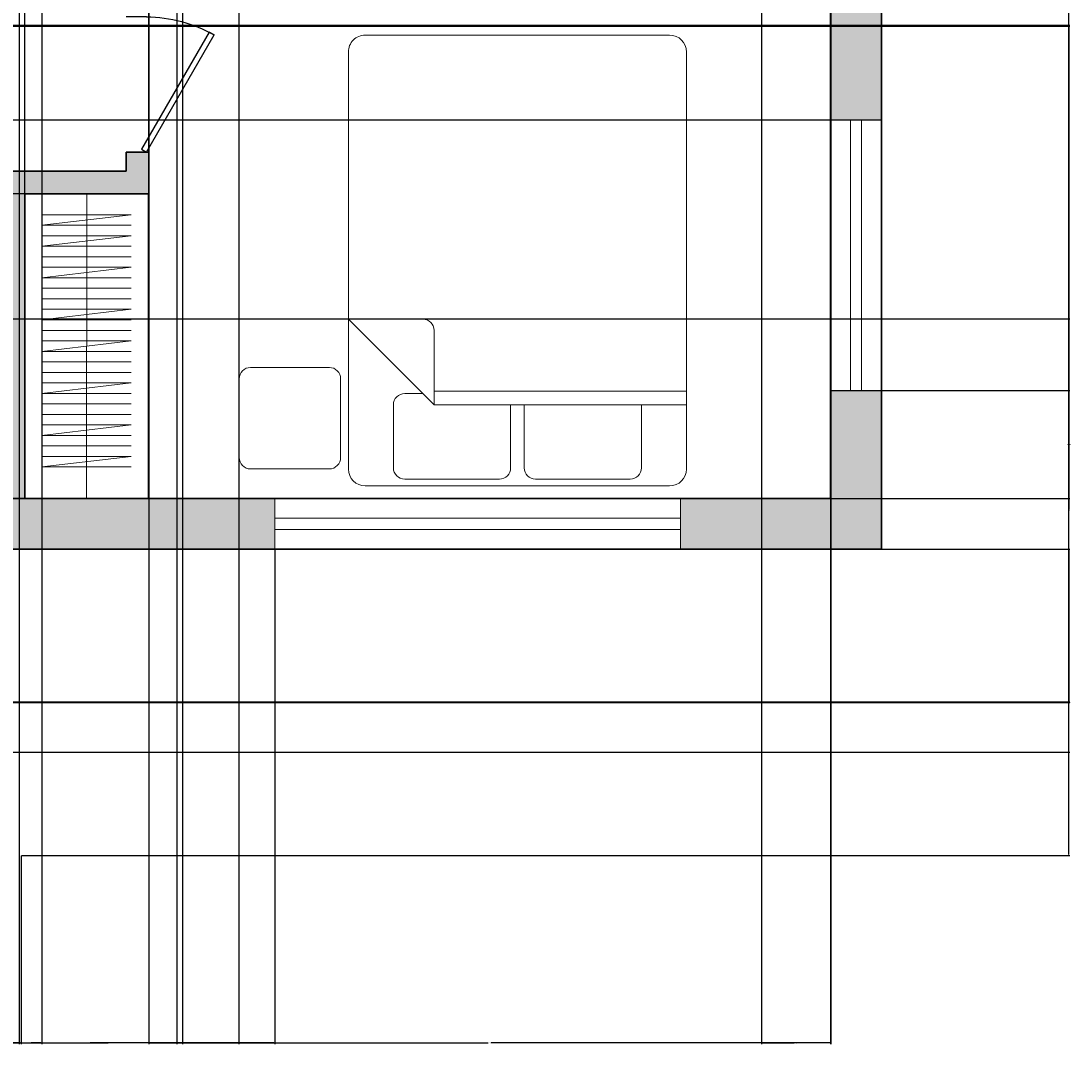
# Model space of a CAD drawing. Units: inches. Extents: x 1531 to 2263, y 2711 to 3216.
# Tile 9 of 12: x 2076 to 2263, y 2711 to 2893. Entities that reach past the tile are written whole.
import ezdxf

# ---------------------------------------------------------------- set-up
doc = ezdxf.new("R2010")
doc.units = ezdxf.units.IN
for name, color, linetype, lineweight in [('A-ANNO-DIMS', 2, 'Continuous', 18), ('A-DOOR', 3, 'Continuous', 25), ('A-FLOR-CASE', 9, 'Continuous', 18), ('A-FURN', 8, 'Continuous', 18), ('A-GLAZ', 4, 'Continuous', 18), ('A-WALL', 7, 'Continuous', 35)]:
    doc.layers.add(name, color=color, linetype=linetype, lineweight=lineweight)
doc.layers.add('A-WALL-PATT', color=18, linetype='Continuous', lineweight=13, true_color=0x000000)
doc.styles.get("Standard").update_dxf_attribs({"font": 'arial.ttf'})
doc.dimstyles.get("Standard").update_dxf_attribs({"dimtxt": 0.18, "dimasz": 0.18, "dimexe": 0.18, "dimexo": 0.0625, "dimgap": 0.09, "dimtad": 0, "dimtih": 1, "dimtoh": 1, "dimdec": 4, "dimzin": 0, "dimdsep": 46, "dimtxsty": 'Standard', "dimcen": 0.09, "dimadec": 0, "dimazin": 0, "dimtfac": 1, "dimtdec": 4, "dimtofl": 0, "dimtmove": 0, "dimatfit": 3, "dimfxl": 1, "dimtolj": 1, "dimtzin": 0, "dimarcsym": 0})

# ---------------------------------------------------------------- blocks, each defined once
blk = doc.blocks.new('*U3')
for p, q in [((0, 0), (0, -6)), ((40, 0), (40, -6))]:
    blk.add_line(p, q)
blk.add_lwpolyline([(0, 0), (34.64, 20), (35.52, 18.48), (0.87, -1.52)], close=True)
blk.add_arc((0, 0), 40, 0, 30)
blk = doc.blocks.new('Bed - Queen')
for p, q in [((3, 0), (57, 0)), ((10, -1.2), (26.8, -1.2)), ((33.2, -1.2), (50, -1.2)), ((0, -77), (0, -3)), ((8, -14.4), (8, -3.2)), ((28.8, -3.2), (28.8, -14.4)), ((31.2, -14.4), (31.2, -3.2)), ((52, -3.2), (52, -14.4)), ((60, -3), (60, -77)), ((0, -14.4), (44.8, -14.4)), ((60, -29.6), (44.8, -14.4)), ((44.8, -14.4), (44.8, -27.6)), ((50, -16.4), (46.8, -16.4)), ((44.8, -16.8), (0, -16.8)), ((46.8, -29.6), (60, -29.6)), ((57, -80), (3, -80))]:
    blk.add_line(p, q)
blk.add_lwpolyline([(63.37, -3.02), (77.37, -3.02, -0.414214), (79.37, -5.02), (79.37, -19.02, -0.414214), (77.37, -21.02), (63.37, -21.02, -0.414214), (61.37, -19.02), (61.37, -5.02, -0.414214)], format="xyb", close=True)
for centre, radius, start, end in [((3, -3), 3, 90, 180), ((57, -3), 3, 0, 90), ((10, -3.2), 2, 90, 180), ((26.8, -3.2), 2, 0, 90), ((33.2, -3.2), 2, 90, 180), ((50, -3.2), 2, 0, 90), ((50, -14.4), 2, 270, 0), ((46.8, -27.6), 2, 180, 270), ((3, -77), 3, 180, 270), ((57, -77), 3, 270, 0)]:
    blk.add_arc(centre, radius, start, end)
blk = doc.blocks.new('WIN-72IN')
for p, q in [((0, 5.5), (72, 5.5)), ((0, 3.5), (72, 3.5))]:
    blk.add_line(p, q)
for points in [[(0, 9), (0, 0)], [(72, 0), (72, 9)]]:
    blk.add_lwpolyline(points)
blk = doc.blocks.new('WIN-48IN')
for p, q in [((3.5, 48), (3.5, 0)), ((5.5, 48), (5.5, 0))]:
    blk.add_line(p, q)
for points in [[(0, 48), (9, 48)], [(9, 0), (0, 0)]]:
    blk.add_lwpolyline(points)
blk = doc.blocks.new('*D55')
at = {"layer": 'A-ANNO-DIMS', "color": 0, "lineweight": -2, "transparency": 16777216}
for p, q in [((2228.97, 3183.02), (2262.37, 3183.02)), ((2262.19, 3182.84), (2262.19, 2963.95)), ((2262.19, 2744.7), (2262.19, 2963.59)), ((2076.3, 2744.52), (2262.37, 2744.52))]:
    blk.add_line(p, q, dxfattribs=at)
at = {"layer": 'A-ANNO-DIMS', "color": 0, "transparency": 16777216}
for points in [[(2262.16, 3182.84), (2262.22, 3182.84), (2262.19, 3183.02)], [(2262.16, 2744.7), (2262.22, 2744.7), (2262.19, 2744.52)]]:
    blk.add_solid(points, dxfattribs=at)
at = {"layer": 'Defpoints', "color": 0, "transparency": 16777216}
for p in [(2228.91, 3183.02), (2076.24, 2744.52), (2262.19, 2744.52)]:
    blk.add_point(p, dxfattribs=at)
at = {"layer": 'A-ANNO-DIMS', "color": 0, "transparency": 16777216, "insert": (2262.19, 2963.77), "char_height": 0.18, "attachment_point": 5}
blk.add_mtext('\\A1;438.5', dxfattribs=at)
blk = doc.blocks.new('*D65')
at = {"layer": 'A-ANNO-DIMS', "color": 0, "lineweight": -2, "transparency": 16777216}
for p, q in [((1577.97, 2891.68), (2262.37, 2891.68)), ((2262.19, 2891.5), (2262.19, 2831.86)), ((2262.19, 2771.86), (2262.19, 2831.5)), ((1577.97, 2771.68), (2262.37, 2771.68))]:
    blk.add_line(p, q, dxfattribs=at)
at = {"layer": 'A-ANNO-DIMS', "color": 0, "transparency": 16777216}
for points in [[(2262.16, 2891.5), (2262.22, 2891.5), (2262.19, 2891.68)], [(2262.16, 2771.86), (2262.22, 2771.86), (2262.19, 2771.68)]]:
    blk.add_solid(points, dxfattribs=at)
at = {"layer": 'Defpoints', "color": 0, "transparency": 16777216}
for p in [(1577.91, 2891.68), (1577.91, 2771.68), (2262.19, 2771.68)]:
    blk.add_point(p, dxfattribs=at)
at = {"layer": 'A-ANNO-DIMS', "color": 0, "transparency": 16777216, "insert": (2262.19, 2831.68), "char_height": 0.18, "attachment_point": 5}
blk.add_mtext('\\A1;120', dxfattribs=at)
blk = doc.blocks.new('*D70')
at = {"layer": 'A-ANNO-DIMS', "color": 0, "lineweight": -2, "transparency": 16777216}
for p, q in [((1736.97, 2839.76), (2262.37, 2839.76)), ((2262.19, 2839.58), (2262.19, 2805.94)), ((2262.19, 2771.94), (2262.19, 2805.58)), ((1736.97, 2771.76), (2262.37, 2771.76))]:
    blk.add_line(p, q, dxfattribs=at)
at = {"layer": 'A-ANNO-DIMS', "color": 0, "transparency": 16777216}
for points in [[(2262.16, 2839.58), (2262.22, 2839.58), (2262.19, 2839.76)], [(2262.16, 2771.94), (2262.22, 2771.94), (2262.19, 2771.76)]]:
    blk.add_solid(points, dxfattribs=at)
at = {"layer": 'Defpoints', "color": 0, "transparency": 16777216}
for p in [(1736.91, 2839.76), (2262.19, 2839.76), (1736.91, 2771.76)]:
    blk.add_point(p, dxfattribs=at)
at = {"layer": 'A-ANNO-DIMS', "color": 0, "transparency": 16777216, "insert": (2262.19, 2805.76), "char_height": 0.18, "attachment_point": 5}
blk.add_mtext('\\A1;68', dxfattribs=at)
blk = doc.blocks.new('*D72')
at = {"layer": 'A-ANNO-DIMS', "color": 0, "lineweight": -2, "transparency": 16777216}
for p, q in [((1986.65, 2744.45), (1986.65, 2711.06)), ((2076.24, 2744.45), (2076.24, 2711.06)), ((1986.83, 2711.24), (2031.05, 2711.24)), ((2076.06, 2711.24), (2031.84, 2711.24))]:
    blk.add_line(p, q, dxfattribs=at)
at = {"layer": 'A-ANNO-DIMS', "color": 0, "transparency": 16777216}
for points in [[(1986.83, 2711.27), (1986.83, 2711.21), (1986.65, 2711.24)], [(2076.06, 2711.27), (2076.06, 2711.21), (2076.24, 2711.24)]]:
    blk.add_solid(points, dxfattribs=at)
at = {"layer": 'Defpoints', "color": 0, "transparency": 16777216}
for p in [(1986.65, 2744.52), (2076.24, 2744.52), (2076.24, 2711.24)]:
    blk.add_point(p, dxfattribs=at)
at = {"layer": 'A-ANNO-DIMS', "color": 0, "transparency": 16777216, "insert": (2031.44, 2711.24), "char_height": 0.18, "attachment_point": 5}
blk.add_mtext('\\A1;89.59', dxfattribs=at)
blk = doc.blocks.new('*D73')
at = {"layer": 'A-ANNO-DIMS', "color": 0, "lineweight": -2, "transparency": 16777216}
for p, q in [((2076.3, 2798.86), (2262.37, 2798.86)), ((2262.19, 2798.68), (2262.19, 2771.87)), ((2262.19, 2744.7), (2262.19, 2771.51)), ((2076.3, 2744.52), (2262.37, 2744.52))]:
    blk.add_line(p, q, dxfattribs=at)
at = {"layer": 'A-ANNO-DIMS', "color": 0, "transparency": 16777216}
for points in [[(2262.16, 2798.68), (2262.22, 2798.68), (2262.19, 2798.86)], [(2262.16, 2744.7), (2262.22, 2744.7), (2262.19, 2744.52)]]:
    blk.add_solid(points, dxfattribs=at)
at = {"layer": 'Defpoints', "color": 0, "transparency": 16777216}
for p in [(2076.24, 2798.86), (2262.19, 2798.86), (2076.24, 2744.52)]:
    blk.add_point(p, dxfattribs=at)
at = {"layer": 'A-ANNO-DIMS', "color": 0, "transparency": 16777216, "insert": (2262.19, 2771.69), "char_height": 0.18, "attachment_point": 5}
blk.add_mtext('\\A1;54.35', dxfattribs=at)
blk = doc.blocks.new('*D74')
at = {"layer": 'A-ANNO-DIMS', "color": 0, "lineweight": -2, "transparency": 16777216}
for p, q in [((2098.91, 2899.27), (2098.91, 2711.06)), ((2219.91, 2899.33), (2219.91, 2711.06)), ((2099.09, 2711.24), (2159.15, 2711.24)), ((2219.73, 2711.24), (2159.67, 2711.24))]:
    blk.add_line(p, q, dxfattribs=at)
at = {"layer": 'A-ANNO-DIMS', "color": 0, "transparency": 16777216}
for points in [[(2099.09, 2711.27), (2099.09, 2711.21), (2098.91, 2711.24)], [(2219.73, 2711.27), (2219.73, 2711.21), (2219.91, 2711.24)]]:
    blk.add_solid(points, dxfattribs=at)
at = {"layer": 'Defpoints', "color": 0, "transparency": 16777216}
for p in [(2098.91, 2899.33), (2219.91, 2899.4), (2219.91, 2711.24)]:
    blk.add_point(p, dxfattribs=at)
at = {"layer": 'A-ANNO-DIMS', "color": 0, "transparency": 16777216, "insert": (2159.41, 2711.24), "char_height": 0.18, "attachment_point": 5}
blk.add_mtext('\\A1;121', dxfattribs=at)
blk = doc.blocks.new('*D75')
at = {"layer": 'A-ANNO-DIMS', "color": 0, "lineweight": -2, "transparency": 16777216}
for p, q in [((2219.85, 2899.4), (1531.04, 2899.4)), ((1531.22, 2899.22), (1531.22, 2853.81)), ((1531.22, 2808.04), (1531.22, 2853.45)), ((2219.85, 2807.86), (1531.04, 2807.86))]:
    blk.add_line(p, q, dxfattribs=at)
at = {"layer": 'A-ANNO-DIMS', "color": 0, "transparency": 16777216}
for points in [[(1531.19, 2899.22), (1531.25, 2899.22), (1531.22, 2899.4)], [(1531.19, 2808.04), (1531.25, 2808.04), (1531.22, 2807.86)]]:
    blk.add_solid(points, dxfattribs=at)
at = {"layer": 'Defpoints', "color": 0, "transparency": 16777216}
for p in [(1531.22, 2899.4), (2219.91, 2899.4), (2219.91, 2807.86)]:
    blk.add_point(p, dxfattribs=at)
at = {"layer": 'A-ANNO-DIMS', "color": 0, "transparency": 16777216, "insert": (1531.22, 2853.63), "char_height": 0.18, "attachment_point": 5}
blk.add_mtext('\\A1;91.53', dxfattribs=at)
blk = doc.blocks.new('*D81')
at = {"layer": 'A-ANNO-DIMS', "color": 0, "lineweight": -2, "transparency": 16777216}
for p, q in [((1933.97, 2891.87), (2262.37, 2891.87)), ((2262.19, 2891.69), (2262.19, 2850.05)), ((2262.19, 2808.04), (2262.19, 2849.68)), ((1933.97, 2807.86), (2262.37, 2807.86))]:
    blk.add_line(p, q, dxfattribs=at)
at = {"layer": 'A-ANNO-DIMS', "color": 0, "transparency": 16777216}
for points in [[(2262.16, 2891.69), (2262.22, 2891.69), (2262.19, 2891.87)], [(2262.16, 2808.04), (2262.22, 2808.04), (2262.19, 2807.86)]]:
    blk.add_solid(points, dxfattribs=at)
at = {"layer": 'Defpoints', "color": 0, "transparency": 16777216}
for p in [(1933.91, 2891.87), (2262.19, 2891.87), (1933.91, 2807.86)]:
    blk.add_point(p, dxfattribs=at)
at = {"layer": 'A-ANNO-DIMS', "color": 0, "transparency": 16777216, "insert": (2262.19, 2849.86), "char_height": 0.18, "attachment_point": 5}
blk.add_mtext('\\A1;84', dxfattribs=at)
blk = doc.blocks.new('*D84')
at = {"layer": 'A-ANNO-DIMS', "color": 0, "lineweight": -2, "transparency": 16777216}
for p, q in [((2079.91, 3089.28), (2079.91, 2711.06)), ((2103.91, 3089.28), (2103.91, 2711.06)), ((2080.09, 2711.24), (2091.69, 2711.24)), ((2103.73, 2711.24), (2092.13, 2711.24))]:
    blk.add_line(p, q, dxfattribs=at)
at = {"layer": 'A-ANNO-DIMS', "color": 0, "transparency": 16777216}
for points in [[(2080.09, 2711.27), (2080.09, 2711.21), (2079.91, 2711.24)], [(2103.73, 2711.27), (2103.73, 2711.21), (2103.91, 2711.24)]]:
    blk.add_solid(points, dxfattribs=at)
at = {"layer": 'Defpoints', "color": 0, "transparency": 16777216}
for p in [(2079.91, 3089.34), (2103.91, 3089.34), (2103.91, 2711.24)]:
    blk.add_point(p, dxfattribs=at)
at = {"layer": 'A-ANNO-DIMS', "color": 0, "transparency": 16777216, "insert": (2091.91, 2711.24), "char_height": 0.18, "attachment_point": 5}
blk.add_mtext('\\A1;24', dxfattribs=at)
blk = doc.blocks.new('*D97')
at = {"layer": 'A-ANNO-DIMS', "color": 0, "lineweight": -2, "transparency": 16777216}
for p, q in [((2054.91, 2798.8), (2054.91, 2711.06)), ((2121.28, 2798.8), (2121.28, 2711.06)), ((2055.09, 2711.24), (2087.7, 2711.24)), ((2121.09, 2711.24), (2088.49, 2711.24))]:
    blk.add_line(p, q, dxfattribs=at)
at = {"layer": 'A-ANNO-DIMS', "color": 0, "transparency": 16777216}
for points in [[(2055.09, 2711.27), (2055.09, 2711.21), (2054.91, 2711.24)], [(2121.09, 2711.27), (2121.09, 2711.21), (2121.28, 2711.24)]]:
    blk.add_solid(points, dxfattribs=at)
at = {"layer": 'Defpoints', "color": 0, "transparency": 16777216}
for p in [(2054.91, 2798.86), (2121.28, 2798.86), (2054.91, 2711.24)]:
    blk.add_point(p, dxfattribs=at)
at = {"layer": 'A-ANNO-DIMS', "color": 0, "transparency": 16777216, "insert": (2088.09, 2711.24), "char_height": 0.18, "attachment_point": 5}
blk.add_mtext('\\A1;66.36', dxfattribs=at)
blk = doc.blocks.new('*D101')
at = {"layer": 'A-ANNO-DIMS', "color": 0, "lineweight": -2, "transparency": 16777216}
for p, q in [((2228.85, 2918.81), (1531.04, 2918.81)), ((1531.22, 2918.63), (1531.22, 2897.08)), ((1531.22, 2875.18), (1531.22, 2896.72)), ((2228.85, 2875), (1531.04, 2875))]:
    blk.add_line(p, q, dxfattribs=at)
at = {"layer": 'A-ANNO-DIMS', "color": 0, "transparency": 16777216}
for points in [[(1531.19, 2918.63), (1531.25, 2918.63), (1531.22, 2918.81)], [(1531.19, 2875.18), (1531.25, 2875.18), (1531.22, 2875)]]:
    blk.add_solid(points, dxfattribs=at)
at = {"layer": 'Defpoints', "color": 0, "transparency": 16777216}
for p in [(2228.91, 2918.81), (1531.22, 2875), (2228.91, 2875)]:
    blk.add_point(p, dxfattribs=at)
at = {"layer": 'A-ANNO-DIMS', "color": 0, "transparency": 16777216, "insert": (1531.22, 2896.9), "char_height": 0.18, "attachment_point": 5}
blk.add_mtext('\\A1;43.81', dxfattribs=at)
blk = doc.blocks.new('*D102')
at = {"layer": 'A-ANNO-DIMS', "color": 0, "lineweight": -2, "transparency": 16777216}
for p, q in [((2219.97, 2827), (2262.37, 2827)), ((2262.19, 2826.82), (2262.19, 2817.61)), ((2262.19, 2808.04), (2262.19, 2817.25)), ((2219.97, 2807.86), (2262.37, 2807.86))]:
    blk.add_line(p, q, dxfattribs=at)
at = {"layer": 'A-ANNO-DIMS', "color": 0, "transparency": 16777216}
for points in [[(2262.16, 2826.82), (2262.22, 2826.82), (2262.19, 2827)], [(2262.16, 2808.04), (2262.22, 2808.04), (2262.19, 2807.86)]]:
    blk.add_solid(points, dxfattribs=at)
at = {"layer": 'Defpoints', "color": 0, "transparency": 16777216}
for p in [(2219.91, 2827), (2262.19, 2827), (2219.91, 2807.86)]:
    blk.add_point(p, dxfattribs=at)
at = {"layer": 'A-ANNO-DIMS', "color": 0, "transparency": 16777216, "insert": (2262.19, 2817.43), "char_height": 0.18, "attachment_point": 5}
blk.add_mtext('\\A1;19.133', dxfattribs=at)
blk = doc.blocks.new('*D105')
at = {"layer": 'A-ANNO-DIMS', "color": 0, "lineweight": -2, "transparency": 16777216}
for p, q in [((2104.87, 2975.27), (2104.87, 2711.06)), ((2114.87, 2975.27), (2114.87, 2711.06)), ((2105.05, 2711.24), (2109.66, 2711.24)), ((2114.69, 2711.24), (2110.08, 2711.24))]:
    blk.add_line(p, q, dxfattribs=at)
at = {"layer": 'A-ANNO-DIMS', "color": 0, "transparency": 16777216}
for points in [[(2105.05, 2711.27), (2105.05, 2711.21), (2104.87, 2711.24)], [(2114.69, 2711.27), (2114.69, 2711.21), (2114.87, 2711.24)]]:
    blk.add_solid(points, dxfattribs=at)
at = {"layer": 'Defpoints', "color": 0, "transparency": 16777216}
for p in [(2104.87, 2975.33), (2114.87, 2975.33), (2114.87, 2711.24)]:
    blk.add_point(p, dxfattribs=at)
at = {"layer": 'A-ANNO-DIMS', "color": 0, "transparency": 16777216, "insert": (2109.87, 2711.24), "char_height": 0.18, "attachment_point": 5}
blk.add_mtext('\\A1;10', dxfattribs=at)
blk = doc.blocks.new('*D108')
at = {"layer": 'A-ANNO-DIMS', "color": 0, "lineweight": -2, "transparency": 16777216}
for p, q in [((1933.97, 2798.86), (2262.37, 2798.86)), ((2262.19, 2798.68), (2262.19, 2781.05)), ((2262.19, 2763.05), (2262.19, 2780.68)), ((1933.97, 2762.87), (2262.37, 2762.87))]:
    blk.add_line(p, q, dxfattribs=at)
at = {"layer": 'A-ANNO-DIMS', "color": 0, "transparency": 16777216}
for points in [[(2262.16, 2798.68), (2262.22, 2798.68), (2262.19, 2798.86)], [(2262.16, 2763.05), (2262.22, 2763.05), (2262.19, 2762.87)]]:
    blk.add_solid(points, dxfattribs=at)
at = {"layer": 'Defpoints', "color": 0, "transparency": 16777216}
for p in [(1933.91, 2798.86), (2262.19, 2798.86), (1933.91, 2762.87)]:
    blk.add_point(p, dxfattribs=at)
at = {"layer": 'A-ANNO-DIMS', "color": 0, "transparency": 16777216, "insert": (2262.19, 2780.86), "char_height": 0.18, "attachment_point": 5}
blk.add_mtext('\\A1;36', dxfattribs=at)
blk = doc.blocks.new('*D123')
at = {"layer": 'A-ANNO-DIMS', "color": 0, "lineweight": -2, "transparency": 16777216}
for p, q in [((2207.66, 3152.42), (2207.66, 2711.06)), ((2219.92, 3149.95), (2219.92, 2711.06)), ((2207.84, 2711.24), (2213.41, 2711.24)), ((2219.74, 2711.24), (2214.18, 2711.24))]:
    blk.add_line(p, q, dxfattribs=at)
at = {"layer": 'A-ANNO-DIMS', "color": 0, "transparency": 16777216}
for points in [[(2207.84, 2711.27), (2207.84, 2711.21), (2207.66, 2711.24)], [(2219.74, 2711.27), (2219.74, 2711.21), (2219.92, 2711.24)]]:
    blk.add_solid(points, dxfattribs=at)
at = {"layer": 'Defpoints', "color": 0, "transparency": 16777216}
for p in [(2207.66, 3152.48), (2219.92, 3150.02), (2207.66, 2711.24)]:
    blk.add_point(p, dxfattribs=at)
at = {"layer": 'A-ANNO-DIMS', "color": 0, "transparency": 16777216, "insert": (2213.79, 2711.24), "char_height": 0.18, "attachment_point": 5}
blk.add_mtext('\\A1;12.26', dxfattribs=at)
blk = doc.blocks.new('*D124')
at = {"layer": 'A-ANNO-DIMS', "color": 0, "lineweight": -2, "transparency": 16777216}
for p, q in [((2076.91, 2862.01), (2076.91, 3216.47)), ((2077.09, 3216.29), (2087.69, 3216.29)), ((2098.73, 3216.29), (2088.13, 3216.29)), ((2098.91, 2862.01), (2098.91, 3216.47))]:
    blk.add_line(p, q, dxfattribs=at)
at = {"layer": 'A-ANNO-DIMS', "color": 0, "transparency": 16777216}
for points in [[(2077.09, 3216.32), (2077.09, 3216.26), (2076.91, 3216.29)], [(2098.73, 3216.32), (2098.73, 3216.26), (2098.91, 3216.29)]]:
    blk.add_solid(points, dxfattribs=at)
at = {"layer": 'Defpoints', "color": 0, "transparency": 16777216}
for p in [(2076.91, 3216.29), (2076.91, 2861.95), (2098.91, 2861.95)]:
    blk.add_point(p, dxfattribs=at)
at = {"layer": 'A-ANNO-DIMS', "color": 0, "transparency": 16777216, "insert": (2087.91, 3216.29), "char_height": 0.18, "attachment_point": 5}
blk.add_mtext('\\A1;22', dxfattribs=at)
blk = doc.blocks.new('*D125')
at = {"layer": 'A-ANNO-DIMS', "color": 0, "lineweight": -2, "transparency": 16777216}
for p, q in [((2076.85, 2861.95), (1531.04, 2861.95)), ((1531.22, 2861.77), (1531.22, 2835.09)), ((1531.22, 2808.04), (1531.22, 2834.72)), ((2076.85, 2807.86), (1531.04, 2807.86))]:
    blk.add_line(p, q, dxfattribs=at)
at = {"layer": 'A-ANNO-DIMS', "color": 0, "transparency": 16777216}
for points in [[(1531.19, 2861.77), (1531.25, 2861.77), (1531.22, 2861.95)], [(1531.19, 2808.04), (1531.25, 2808.04), (1531.22, 2807.86)]]:
    blk.add_solid(points, dxfattribs=at)
at = {"layer": 'Defpoints', "color": 0, "transparency": 16777216}
for p in [(2076.91, 2861.95), (1531.22, 2807.86), (2076.91, 2807.86)]:
    blk.add_point(p, dxfattribs=at)
at = {"layer": 'A-ANNO-DIMS', "color": 0, "transparency": 16777216, "insert": (1531.22, 2834.91), "char_height": 0.18, "attachment_point": 5}
blk.add_mtext('\\A1;54.09', dxfattribs=at)
blk = doc.blocks.new('*D130')
at = {"layer": 'A-ANNO-DIMS', "color": 0, "lineweight": -2, "transparency": 16777216}
for p, q in [((2075.91, 3029.88), (2075.91, 2711.06)), ((2079.91, 3025.88), (2079.91, 2711.06)), ((2076.09, 2711.24), (2077.76, 2711.24)), ((2079.73, 2711.24), (2078.06, 2711.24))]:
    blk.add_line(p, q, dxfattribs=at)
at = {"layer": 'A-ANNO-DIMS', "color": 0, "transparency": 16777216}
for points in [[(2076.09, 2711.27), (2076.09, 2711.21), (2075.91, 2711.24)], [(2079.73, 2711.27), (2079.73, 2711.21), (2079.91, 2711.24)]]:
    blk.add_solid(points, dxfattribs=at)
at = {"layer": 'Defpoints', "color": 0, "transparency": 16777216}
for p in [(2075.91, 3029.94), (2079.91, 3025.94), (2075.91, 2711.24)]:
    blk.add_point(p, dxfattribs=at)
at = {"layer": 'A-ANNO-DIMS', "color": 0, "transparency": 16777216, "insert": (2077.91, 2711.24), "char_height": 0.18, "attachment_point": 5}
blk.add_mtext('\\A1;4', dxfattribs=at)

msp = doc.modelspace()

# ---------------------------------------------------------------- hatches: boundary and pattern name
at = {"layer": 'A-WALL-PATT'}
h = msp.add_hatch(color=256, dxfattribs=at)
h.dxf.hatch_style = 1
h.paths.add_polyline_path([(2228.9101, 2918.8056), (2219.9101, 2918.8056), (2219.9101, 2903.3968), (2213.9101, 2903.3937), (2213.9101, 2899.3968), (2219.9101, 2899.3968), (2219.9101, 2874.9957), (2228.9101, 2874.9957)])
h = msp.add_hatch(color=256, dxfattribs=at)
h.dxf.hatch_style = 1
h.paths.add_polyline_path([(2121.275, 2807.8631), (2076.9101, 2807.8631), (2076.9101, 2861.9499), (2098.9101, 2861.9499), (2098.9101, 2869.3336), (2094.9101, 2869.3336), (2094.9101, 2865.9499), (2072.9101, 2865.9499), (2072.9101, 2807.8631), (2054.9101, 2807.8631), (2054.9101, 2798.8631), (2121.275, 2798.8631)])
h = msp.add_hatch(color=256, dxfattribs=at)
h.dxf.hatch_style = 1
h.paths.add_polyline_path([(2228.9101, 2826.9957), (2219.9101, 2826.9957), (2219.9101, 2807.8631), (2193.275, 2807.8631), (2193.275, 2798.8631), (2228.9101, 2798.8631)])

# ---------------------------------------------------------------- linework, layer by layer
at = {"layer": 'A-FLOR-CASE'}
for p, q in [((2076.9101, 2861.9499), (2098.7759, 2861.9499)), ((2076.9101, 2807.8631), (2076.9101, 2861.9499)), ((2087.9101, 2861.9499), (2087.843, 2807.8631)), ((2098.7759, 2861.9499), (2098.7759, 2807.8631)), ((2076.905, 2860.0848), (2076.9101, 2860.0848)), ((2076.8998, 2858.2197), (2076.9101, 2858.2197)), ((2079.9101, 2858.2197), (2095.7759, 2858.2197)), ((2095.7759, 2858.2197), (2079.9101, 2856.3545)), ((2076.8946, 2856.3545), (2076.9101, 2856.3545)), ((2079.9101, 2856.3545), (2095.7759, 2856.3545)), ((2079.9101, 2854.4894), (2095.7759, 2854.4894)), ((2095.7759, 2854.4894), (2079.9101, 2852.6243)), ((2079.9101, 2852.6243), (2095.7759, 2852.6243)), ((2079.9101, 2850.7591), (2095.7759, 2850.7591)), ((2079.9101, 2848.894), (2095.7759, 2848.894)), ((2095.7759, 2848.894), (2079.9101, 2847.0289)), ((2079.9101, 2847.0289), (2095.7759, 2847.0289)), ((2079.9101, 2845.1637), (2095.7759, 2845.1637)), ((2079.9101, 2843.2986), (2095.7759, 2843.2986)), ((2079.9101, 2841.4335), (2095.7759, 2841.4335)), ((2095.7759, 2841.4335), (2079.9101, 2839.5683)), ((2079.9101, 2839.5683), (2095.7759, 2839.5683)), ((2079.9101, 2837.7032), (2095.7759, 2837.7032)), ((2079.9101, 2835.838), (2095.7759, 2835.838)), ((2095.7759, 2835.838), (2079.9101, 2833.9729)), ((2079.9101, 2833.9729), (2095.7759, 2833.9729)), ((2079.9101, 2832.1078), (2095.7759, 2832.1078)), ((2079.9101, 2830.2426), (2095.7759, 2830.2426)), ((2079.9101, 2828.3775), (2095.7759, 2828.3775)), ((2095.7759, 2828.3775), (2079.9101, 2826.5124)), ((2079.9101, 2826.5124), (2095.7759, 2826.5124)), ((2079.9101, 2824.6472), (2095.7759, 2824.6472)), ((2079.9101, 2822.7821), (2095.7759, 2822.7821)), ((2079.9101, 2820.917), (2095.7759, 2820.917)), ((2095.7759, 2820.917), (2079.9101, 2819.0518)), ((2079.9101, 2819.0518), (2095.7759, 2819.0518)), ((2079.9101, 2817.1867), (2095.7759, 2817.1867)), ((2079.9101, 2815.3216), (2095.7759, 2815.3216)), ((2095.7759, 2815.3216), (2079.9101, 2813.4564)), ((2079.9101, 2813.4564), (2095.7759, 2813.4564)), ((2098.7759, 2807.8631), (2076.9101, 2807.8631))]:
    msp.add_line(p, q, dxfattribs=at)
at = {"layer": 'A-WALL'}
for p, q in [((2219.9101, 2899.3968), (2219.9101, 2807.8631)), ((2098.9101, 2869.3336), (2094.9101, 2869.3336)), ((2094.9101, 2869.3336), (2094.9101, 2865.9499)), ((2098.9101, 2869.3336), (2098.9101, 2861.9499)), ((2094.9258, 2865.9499), (2072.9101, 2865.9499)), ((2094.9101, 2865.9499), (2094.9248, 2865.9499)), ((2094.9237, 2865.9499), (2094.9248, 2865.9499)), ((2098.9101, 2865.952), (2098.9237, 2865.952)), ((2098.9101, 2861.9499), (2076.9101, 2861.9499)), ((2076.9101, 2861.9499), (2076.9101, 2807.8631)), ((2098.9101, 2861.952), (2098.9258, 2861.952)), ((2076.9101, 2807.8631), (2219.9101, 2807.8631)), ((2054.9101, 2798.8631), (2228.9101, 2798.8631))]:
    msp.add_line(p, q, dxfattribs=at)
msp.add_lwpolyline([(1933.9101, 2762.8657), (1568.9111, 2762.6748), (1568.9111, 3182.6749), (2228.9101, 3183.02), (2228.9101, 2798.8631)], dxfattribs=at)

# ---------------------------------------------------------------- block references
at = {"layer": 'A-DOOR', "xscale": -0.6, "yscale": 0.6, "zscale": 0.6, "rotation": 270}
msp.add_blockref('*U3', (2098.5101, 2869.3336), dxfattribs=at)
at = {"layer": 'A-FURN', "rotation": 180}
msp.add_blockref('Bed - Queen', (2194.3244, 2810.0977), dxfattribs=at)
at = {"layer": 'A-GLAZ'}
for name, p in [('WIN-48IN', (2219.9101, 2826.9962)), ('WIN-72IN', (2121.2751, 2798.8631))]:
    msp.add_blockref(name, p, dxfattribs=at)

# ---------------------------------------------------------------- dimensions: what is measured, and where the dimension line sits
at = {"layer": 'A-ANNO-DIMS'}
for base, p1, p2, override, picture, middle in [((2076.9101, 3216.295), (2098.9101, 2861.9499), (2076.9101, 2861.9499), {"dimdec": 0, "dimlfac": 1, "dimrnd": 0, "dimzin": 0, "dimdsep": 46, "dimlunit": 2}, '*D124', (2087.9101, 3216.295)), ((2207.6621, 2711.2407), (2219.9227, 3150.0153), (2207.6621, 3152.4778), {"dimdec": 2, "dimlfac": 1, "dimrnd": 0, "dimzin": 0, "dimdsep": 46, "dimlunit": 2}, '*D123', (2213.7924, 2711.2407)), ((2103.9101, 2711.2407), (2079.9101, 3089.343), (2103.9101, 3089.343), {"dimdec": 0, "dimlfac": 1, "dimrnd": 0, "dimzin": 0, "dimdsep": 46, "dimlunit": 2}, '*D84', (2091.9101, 2711.2407)), ((2075.9101, 2711.2407), (2079.9101, 3025.9421), (2075.9101, 3029.94), {"dimdec": 0, "dimlfac": 1, "dimrnd": 0, "dimzin": 0, "dimdsep": 46, "dimlunit": 2}, '*D130', (2077.9101, 2711.2407)), ((2114.8725, 2711.2407), (2104.8725, 2975.3315), (2114.8725, 2975.3315), {"dimdec": 0, "dimlfac": 1, "dimrnd": 0, "dimzin": 0, "dimdsep": 46, "dimlunit": 2}, '*D105', (2109.8725, 2711.2407)), ((2219.9101, 2711.2407), (2098.9101, 2899.3336), (2219.9101, 2899.3968), {"dimdec": 0, "dimlfac": 1, "dimrnd": 0, "dimzin": 0, "dimdsep": 46, "dimlunit": 2}, '*D74', (2159.4101, 2711.2407)), ((2054.9101, 2711.2407), (2121.275, 2798.8631), (2054.9101, 2798.8631), {"dimdec": 2, "dimlfac": 1, "dimrnd": 0, "dimzin": 0, "dimdsep": 46, "dimlunit": 2}, '*D97', (2088.0926, 2711.2407)), ((2076.2365, 2711.2407), (1986.6484, 2744.5157), (2076.2365, 2744.5157), {"dimdec": 2, "dimlfac": 1, "dimrnd": 0, "dimzin": 0, "dimdsep": 46, "dimlunit": 2}, '*D72', (2031.4424, 2711.2407))]:
    dim = msp.add_linear_dim(base=base, p1=p1, p2=p2, dimstyle='Standard', override=override, dxfattribs=at)
    dim.commit()
    dim.dimension.update_dxf_attribs({"geometry": picture, "text_midpoint": middle})
for base, p1, p2, override, picture, middle in [((2262.1851, 2744.5157), (2228.9101, 3183.02), (2076.2365, 2744.5157), {"dimdec": 1, "dimlfac": 1, "dimrnd": 0, "dimzin": 0, "dimdsep": 46, "dimlunit": 2}, '*D55', (2262.1851, 2963.7678)), ((1531.2212, 2874.9957), (2228.9101, 2918.8056), (2228.9101, 2874.9957), {"dimdec": 2, "dimlfac": 1, "dimrnd": 0, "dimzin": 0, "dimdsep": 46, "dimlunit": 2}, '*D101', (1531.2212, 2896.9007)), ((1531.2212, 2899.3968), (2219.9101, 2807.8631), (2219.9101, 2899.3968), {"dimdec": 2, "dimlfac": 1, "dimrnd": 0, "dimzin": 0, "dimdsep": 46, "dimlunit": 2}, '*D75', (1531.2212, 2853.63)), ((2262.1851, 2891.8657), (1933.9101, 2807.8631), (1933.9101, 2891.8657), {"dimdec": 0, "dimlfac": 1, "dimrnd": 0, "dimzin": 0, "dimdsep": 46, "dimlunit": 2}, '*D81', (2262.1851, 2849.8644)), ((2262.1851, 2771.6796), (1577.9111, 2891.6796), (1577.9111, 2771.6796), {"dimdec": 0, "dimlfac": 1, "dimrnd": 0, "dimzin": 0, "dimdsep": 46, "dimlunit": 2}, '*D65', (2262.1851, 2831.6796)), ((1531.2212, 2807.8631), (2076.9101, 2861.9499), (2076.9101, 2807.8631), {"dimdec": 2, "dimlfac": 1, "dimrnd": 0, "dimzin": 0, "dimdsep": 46, "dimlunit": 2}, '*D125', (1531.2212, 2834.9065)), ((2262.1851, 2839.7627), (1736.9101, 2771.7627), (1736.9101, 2839.7627), {"dimdec": 0, "dimlfac": 1, "dimrnd": 0, "dimzin": 0, "dimdsep": 46, "dimlunit": 2}, '*D70', (2262.1851, 2805.7627)), ((2262.1851, 2826.9957), (2219.9101, 2807.8631), (2219.9101, 2826.9957), {"dimdec": 3, "dimlfac": 1, "dimrnd": 0, "dimzin": 0, "dimdsep": 46, "dimlunit": 2}, '*D102', (2262.1851, 2817.4294)), ((2262.1851, 2798.8631), (1933.9101, 2762.8657), (1933.9101, 2798.8631), {"dimdec": 0, "dimlfac": 1, "dimrnd": 0, "dimzin": 0, "dimdsep": 46, "dimlunit": 2}, '*D108', (2262.1851, 2780.8644)), ((2262.1851, 2798.8631), (2076.2365, 2744.5157), (2076.2365, 2798.8631), {"dimdec": 2, "dimlfac": 1, "dimrnd": 0, "dimzin": 0, "dimdsep": 46, "dimlunit": 2}, '*D73', (2262.1851, 2771.6894))]:
    dim = msp.add_linear_dim(base=base, p1=p1, p2=p2, angle=90, dimstyle='Standard', override=override, dxfattribs=at)
    dim.commit()
    dim.dimension.update_dxf_attribs({"geometry": picture, "text_midpoint": middle})

doc.saveas('drawing.dxf')
